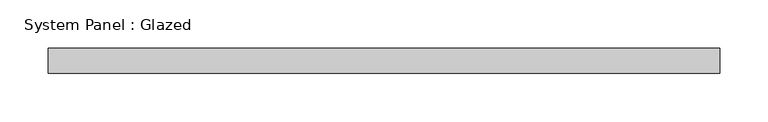
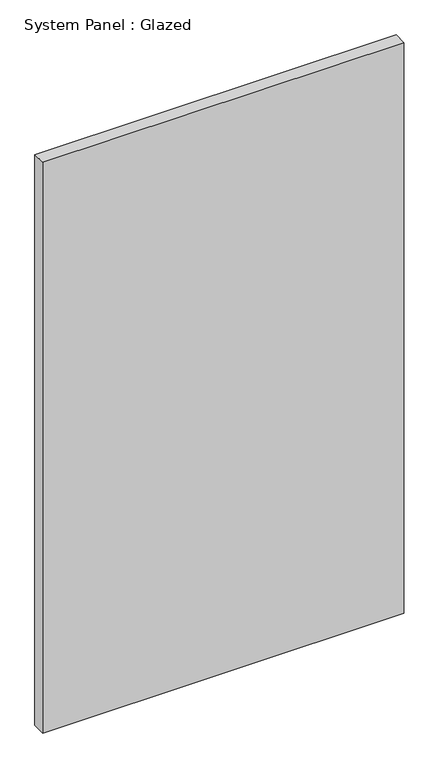
"""IFC4 building model written with IfcOpenShell, lengths in millimetres: plate geometry, System Panel : Glazed."""

from ifc_helpers import new_model, si_unit, origin, origin_with_axes, place, context, project, spatial, polyline, outline, extrude, source, transform, mapped, element, save


def system_panel_glazed_5b6ac675(model_context):
    return source(origin(), model_context, "Body", "SweptSolid", [
        extrude(outline(polyline([(345.9730186, 19.05), (-345.9730186, 19.05), (-345.9730186, 44.45), (345.9730186, 44.45), (345.9730186, 19.05)])), origin_with_axes(), (0.0, 0.0, 1.0), 1155.7),
    ])


if __name__ == "__main__":
    model = new_model("IFC4")
    model_context = context("Model", 3, world=origin())
    ifc_project = project(units=[si_unit("LENGTHUNIT", "METRE", prefix="MILLI")], contexts=[model_context])
    site = spatial("IfcSite", under=ifc_project)
    building = spatial("IfcBuilding", under=site)
    placement = place(None, origin())
    system_panel_glazed_shape = system_panel_glazed_5b6ac675(model_context)
    element("IfcPlate", 1, ObjectType="System Panel : Glazed", at=placement, inside=building, context=model_context, shape_type="MappedRepresentation", body=[
        mapped(system_panel_glazed_shape, transform((0.0, 0.0, 0.0), x_axis=(1.0, 0.0, 0.0), y_axis=(0.0, 1.0, 0.0), z_axis=(0.0, 0.0, 1.0))),
    ])
    save(model, "model.ifc")

# Revit data of these elements
# Type "System Panel : Glazed"
#   Construction Type Id = "GSP4R"
#   Analytic Construction = "1/8 in Pilkington single glazing"
#   Visual Light Transmittance = 0.9
#   Solar Heat Gain Coefficient = 0.86
#   Heat Transfer Coefficient (U) = 1.18115 BTU/(h·ft²·°F)
# Element 1 (IfcPlate, "System Panel : Glazed")
#   Materials on its faces: "Glass"
# Materials
#   "Glass": class "Glass", colour RGB 0 128 192, transparency 0.75, Description = "Soda Lime Glass", Cost = 0
